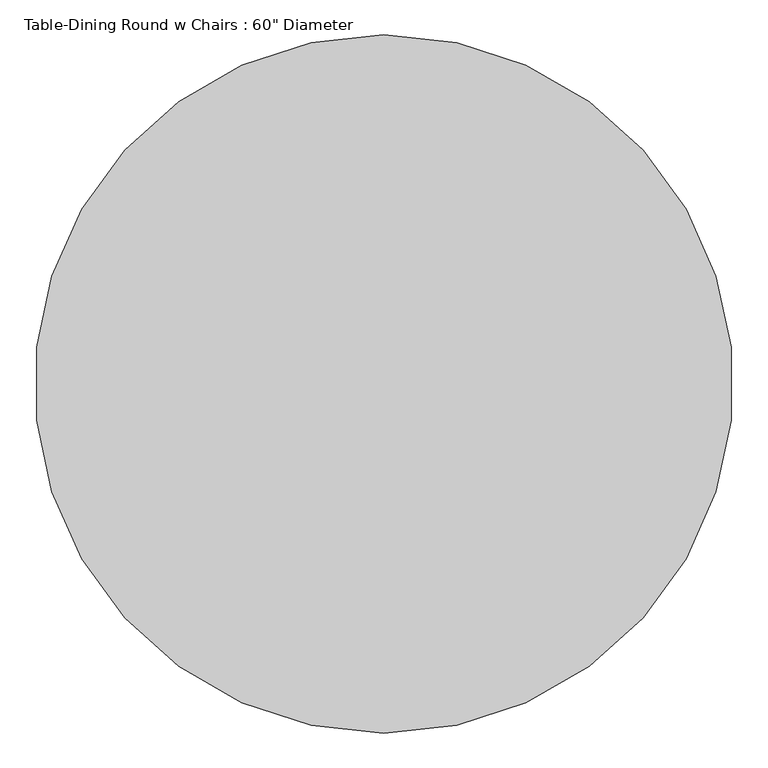
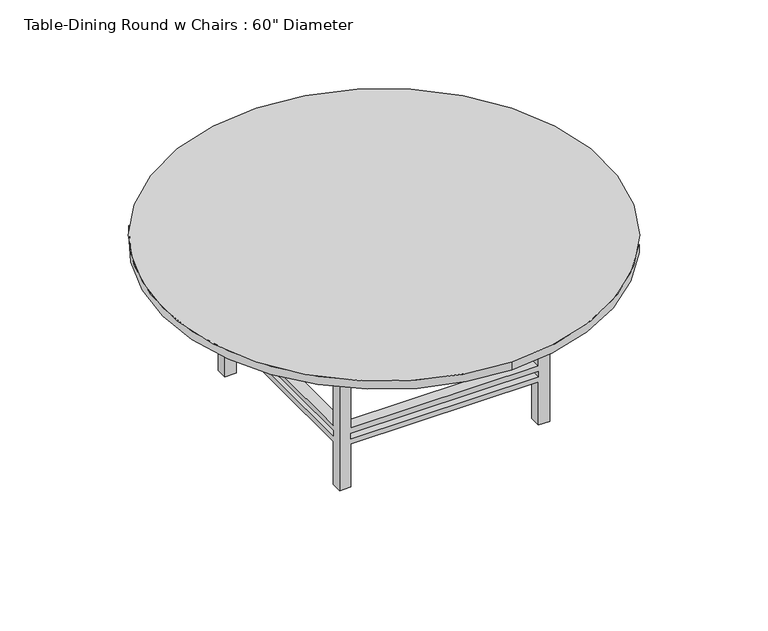
"""IFC4 building model written with IfcOpenShell, lengths in millimetres: furniture geometry."""

from ifc_helpers import new_model, si_unit, point, frame, frame_2d, origin, place, context, project, spatial, polyline, circle_curve, trimmed, segment, composite_curve, outline, extrude, faceted_brep, source, transform, mapped, element, save


def furniture_7cf74a4d(model_context):
    return source(origin(), model_context, "Body", "SolidModel", [
        faceted_brep([(522.7819672, 234.2213115, 279.4), (522.7819672, -603.9786885, 279.4), (573.5819672, -603.9786885, 279.4), (573.5819672, 234.2213115, 279.4), (-315.4180328, -603.9786885, 279.4), (-315.4180328, -654.7786885, 279.4), (522.7819672, -654.7786885, 279.4), (-315.4180328, 234.2213115, 279.4), (-366.2180328, 234.2213115, 279.4), (-366.2180328, -603.9786885, 279.4), (522.7819672, 285.0213115, 279.4), (-315.4180328, 285.0213115, 279.4), (522.7819672, 234.2213115, 254.0), (-315.4180328, 234.2213115, 254.0), (-315.4180328, 285.0213115, 254.0), (522.7819672, 285.0213115, 254.0), (-315.4180328, -603.9786885, 254.0), (-366.2180328, -603.9786885, 254.0), (-366.2180328, 234.2213115, 254.0), (522.7819672, -603.9786885, 254.0), (522.7819672, -654.7786885, 254.0), (-315.4180328, -654.7786885, 254.0), (573.5819672, 234.2213115, 254.0), (573.5819672, -603.9786885, 254.0), (-366.2180328, 285.0213115, 647.7), (-315.4180328, 285.0213115, 647.7), (522.7819672, 285.0213115, 647.7), (573.5819672, 285.0213115, 647.7), (573.5819672, 285.0213115, 0.0), (522.7819672, 285.0213115, 0.0), (522.7819672, 285.0213115, 203.2), (-315.4180328, 285.0213115, 203.2), (-315.4180328, 285.0213115, 0.0), (-366.2180328, 285.0213115, 0.0), (-315.4180328, 285.0213115, 228.6), (522.7819672, 285.0213115, 228.6), (-366.2180328, 234.2213115, 647.7), (-366.2180328, 234.2213115, 0.0), (-366.2180328, 234.2213115, 203.2), (-366.2180328, -603.9786885, 203.2), (-366.2180328, -603.9786885, 0.0), (-366.2180328, -654.7786885, 0.0), (-366.2180328, -654.7786885, 647.7), (-366.2180328, -603.9786885, 647.7), (-366.2180328, -603.9786885, 228.6), (-366.2180328, 234.2213115, 228.6), (573.5819672, -654.7786885, 647.7), (522.7819672, -654.7786885, 647.7), (-315.4180328, -654.7786885, 647.7), (-315.4180328, -654.7786885, 0.0), (-315.4180328, -654.7786885, 203.2), (522.7819672, -654.7786885, 203.2), (522.7819672, -654.7786885, 0.0), (573.5819672, -654.7786885, 0.0), (522.7819672, -654.7786885, 228.6), (-315.4180328, -654.7786885, 228.6), (573.5819672, 234.2213115, 647.7), (573.5819672, -603.9786885, 647.7), (573.5819672, -603.9786885, 0.0), (573.5819672, -603.9786885, 203.2), (573.5819672, 234.2213115, 203.2), (573.5819672, 234.2213115, 0.0), (573.5819672, 234.2213115, 228.6), (573.5819672, -603.9786885, 228.6), (-315.4180328, 234.2213115, 647.7), (522.7819672, -603.9786885, 647.7), (522.7819672, 234.2213115, 647.7), (-315.4180328, -603.9786885, 647.7), (522.7819672, 234.2213115, 0.0), (-315.4180328, -603.9786885, 0.0), (-315.4180328, 234.2213115, 0.0), (522.7819672, -603.9786885, 0.0), (-315.4180328, 234.2213115, 228.6), (-315.4180328, 234.2213115, 203.2), (522.7819672, 234.2213115, 228.6), (522.7819672, 234.2213115, 203.2), (522.7819672, -603.9786885, 228.6), (522.7819672, -603.9786885, 203.2), (-315.4180328, -603.9786885, 228.6), (-315.4180328, -603.9786885, 203.2)], [[[0, 1, 2, 3]], [[1, 4, 5, 6]], [[4, 7, 8, 9]], [[7, 0, 10, 11]], [[12, 13, 14, 15]], [[13, 16, 17, 18]], [[16, 19, 20, 21]], [[19, 12, 22, 23]], [[24, 25, 11, 10, 26, 27, 28, 29, 30, 31, 32, 33], [14, 34, 35, 15]], [[36, 24, 33, 37, 38, 39, 40, 41, 42, 43, 9, 8], [17, 44, 45, 18]], [[46, 47, 6, 5, 48, 42, 41, 49, 50, 51, 52, 53], [20, 54, 55, 21]], [[28, 27, 56, 3, 2, 57, 46, 53, 58, 59, 60, 61], [22, 62, 63, 23]], [[1, 0, 12, 19]], [[4, 1, 19, 16]], [[7, 4, 16, 13]], [[0, 7, 13, 12]], [[25, 24, 36, 64]], [[47, 46, 57, 65]], [[26, 66, 56, 27]], [[48, 67, 43, 42]], [[29, 28, 61, 68]], [[49, 41, 40, 69]], [[32, 70, 37, 33]], [[52, 71, 58, 53]], [[13, 18, 45, 72]], [[64, 36, 8, 7]], [[37, 70, 73, 38]], [[14, 13, 72, 34]], [[25, 64, 7, 11]], [[70, 32, 31, 73]], [[12, 15, 35, 74]], [[66, 26, 10, 0]], [[29, 68, 75, 30]], [[22, 12, 74, 62]], [[56, 66, 0, 3]], [[68, 61, 60, 75]], [[19, 23, 63, 76]], [[65, 57, 2, 1]], [[58, 71, 77, 59]], [[20, 19, 76, 54]], [[47, 65, 1, 6]], [[71, 52, 51, 77]], [[16, 21, 55, 78]], [[67, 48, 5, 4]], [[49, 69, 79, 50]], [[17, 16, 78, 44]], [[43, 67, 4, 9]], [[69, 40, 39, 79]], [[74, 76, 63, 62]], [[76, 78, 55, 54]], [[78, 72, 45, 44]], [[72, 74, 35, 34]], [[75, 73, 31, 30]], [[73, 79, 39, 38]], [[79, 77, 51, 50]], [[77, 75, 60, 59]], [[76, 74, 75, 77]], [[78, 76, 77, 79]], [[72, 78, 79, 73]], [[74, 72, 73, 75]]]),
        extrude(outline(polyline([(598.9819672, 310.4213115), (598.9819672, -680.1786885), (-391.6180328, -680.1786885), (-391.6180328, 310.4213115), (598.9819672, 310.4213115)]), holes=[polyline([(573.5819672, 285.0213115), (-366.2180328, 285.0213115), (-366.2180328, -654.7786885), (573.5819672, -654.7786885), (573.5819672, 285.0213115)])]), frame((0.0, 0.0, 647.7), z_axis=(0.0, 0.0, 1.0), x_axis=(1.0, 0.0, 0.0)), (0.0, 0.0, 1.0), 76.2),
        extrude(outline(composite_curve([segment(trimmed(circle_curve(frame_2d((103.6819672, -184.8786885)), 990.6), [point((103.6819672, -1175.4786885))], [point((103.6819672, 805.7213115))], False, "CARTESIAN"), True, "CONTINUOUS"), segment(trimmed(circle_curve(frame_2d((103.6819672, -184.8786885)), 990.6), [point((103.6819672, 805.7213115))], [point((103.6819672, -1175.4786885))], False, "CARTESIAN"), True, "CONTINUOUS")], self_intersect=False)), frame((0.0, 0.0, 723.9), z_axis=(0.0, 0.0, 1.0), x_axis=(1.0, 0.0, 0.0)), (0.0, 0.0, 1.0), 38.1),
    ])


if __name__ == "__main__":
    model = new_model("IFC4")
    model_context = context("Model", 3, world=origin())
    ifc_project = project(units=[si_unit("LENGTHUNIT", "METRE", prefix="MILLI")], contexts=[model_context])
    site = spatial("IfcSite", under=ifc_project)
    building = spatial("IfcBuilding", under=site)
    placement = place(None, origin())
    furniture_shape = furniture_7cf74a4d(model_context)
    element("IfcFurniture", 1, ObjectType="Table-Dining Round w Chairs : 60\" Diameter", at=placement, inside=building, context=model_context, shape_type="MappedRepresentation", body=[
        mapped(furniture_shape, transform((0.0, 0.0, 0.0), x_axis=(1.0, 0.0, 0.0), y_axis=(0.0, 1.0, 0.0), z_axis=(0.0, 0.0, 1.0))),
    ])
    save(model, "model.ifc")

# Revit data of these elements
# Type "Table-Dining Round w Chairs : 60\" Diameter"
#   Assembly Code = "E2020200"
#   Radius = 3' - 3"
#   Diameter = 6' - 6"
#   Height = 2' - 6"
#   Chairs = 10
#   Base Material = Pine
#   Top Material = Laminate, Linen, Matte
#   Default Elevation = 0
# Element 1 (IfcFurniture, "Table-Dining Round w Chairs : 60\" Diameter")
#   Materials on its faces: "Pine", "Laminate, Linen, Matte"
# Materials
#   "Pine": class "Wood", colour RGB 223 192 134, transparency 0, Description = "Pinus Echinata", Cost = 0
#   "Laminate, Linen, Matte": class "Plastic", colour RGB 249 239 230, transparency 0, Description = "Plastic Laminate - Linen, Matte", Cost = 0
